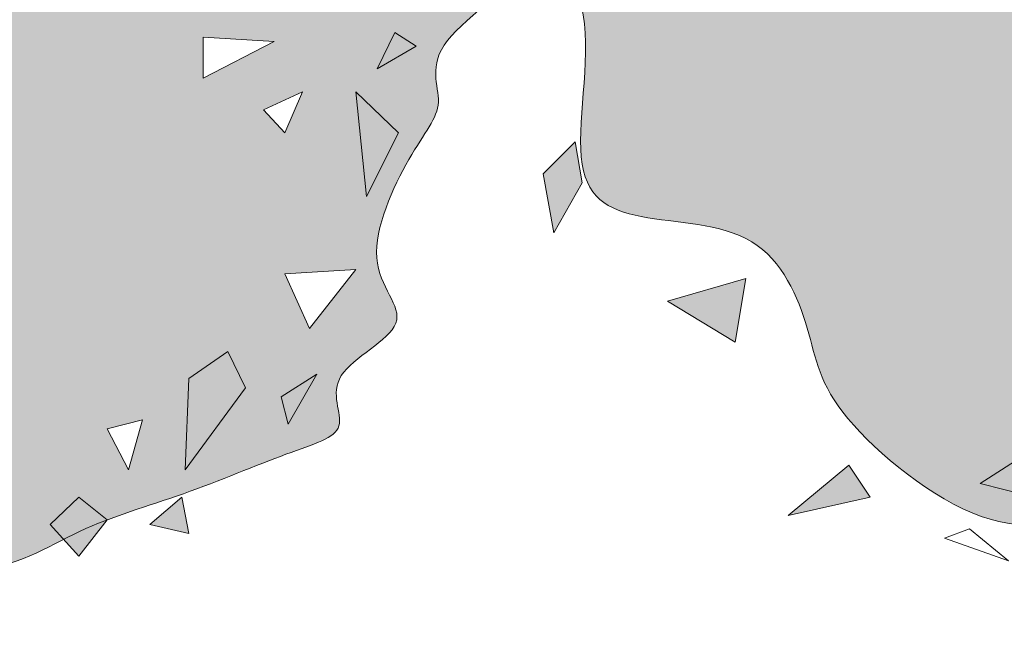
# Model space of a CAD drawing. Units: metres. Extents: x 4298.5 to 4325.2, y 2075 to 2095.8.
# Tile 6 of 35: x 4306.6693 to 4307.1445, y 2079.0337 to 2079.3365. Entities that reach past the tile are written whole.
import ezdxf

# ---------------------------------------------------------------- set-up
doc = ezdxf.new("R2010")
doc.units = ezdxf.units.M
doc.layers.add('A-ANNO-DIMS', color=2, linetype='Continuous', lineweight=18)
doc.layers.add('L-PLNT', color=94, linetype='Continuous', lineweight=13)
doc.layers.add('L-PLNT-PATT', color=116, linetype='Continuous', lineweight=13, true_color=0x13823e)
doc.styles.get("Standard").update_dxf_attribs({"font": 'arial.ttf'})
doc.dimstyles.get("Standard").update_dxf_attribs({"dimtxt": 0.18, "dimasz": 0.18, "dimexe": 0.18, "dimexo": 0.0625, "dimgap": 0.09, "dimtad": 0, "dimtih": 1, "dimtoh": 1, "dimdec": 4, "dimzin": 0, "dimdsep": 46, "dimtxsty": 'Standard', "dimcen": 0.09, "dimadec": 0, "dimazin": 0, "dimtfac": 1, "dimtdec": 4, "dimtofl": 0, "dimtmove": 0, "dimatfit": 3, "dimfxl": 1, "dimtolj": 1, "dimtzin": 0, "dimarcsym": 0})

# ---------------------------------------------------------------- blocks, each defined once
blk = doc.blocks.new('*U9')
for points in [[(7.783, -0.803), (6.433, -1.495), (6.433, -0.716)], [(10.078, -0.629), (9.74, -1.322), (10.482, -0.889)], [(8.323, -1.754), (7.985, -2.533), (7.581, -2.1)], [(9.335, -1.754), (9.538, -3.744), (10.145, -2.533)], [(-10.034, -2.706), (-10.641, -3.312), (-10.439, -4.436), (-9.899, -3.485)], [(9.335, -5.129), (8.458, -6.253), (7.985, -5.215)], [(-8.279, -5.734), (-6.794, -5.302), (-6.997, -6.513)], [(6.096, -8.935), (6.163, -7.205), (6.906, -6.686), (7.243, -7.378)], [(8.053, -8.07), (8.593, -7.118), (7.918, -7.551)], [(5.286, -7.984), (4.611, -8.157), (5.016, -8.935)], [(-2.34, -9.195), (-1.26, -8.503), (-0.99, -9.541)], [(-4.837, -8.849), (-4.432, -9.454), (-5.985, -9.801)], [(4.071, -9.454), (3.531, -9.974), (4.071, -10.579), (4.611, -9.887)], [(6.028, -9.454), (5.421, -9.974), (6.163, -10.147)], [(-2.543, -10.06), (-3.015, -10.233), (-1.8, -10.666)]]:
    blk.add_lwpolyline(points, close=True)
blk = doc.blocks.new('*D23')
at = {"layer": 'A-ANNO-DIMS', "color": 0, "lineweight": -2, "transparency": 16777216}
for p, q in [((4308.16058, 2079.85556), (4308.16058, 2079.58806)), ((4309.16058, 2079.85556), (4309.16058, 2079.58806)), ((4308.16058, 2079.76806), (4307.98058, 2079.76806)), ((4308.98058, 2079.76806), (4308.34058, 2079.76806))]:
    blk.add_line(p, q, dxfattribs=at)
at = {"layer": 'A-ANNO-DIMS', "color": 0, "transparency": 16777216}
for points in [[(4308.34058, 2079.79806), (4308.34058, 2079.73806), (4308.16058, 2079.76806)], [(4308.98058, 2079.79806), (4308.98058, 2079.73806), (4309.16058, 2079.76806)]]:
    blk.add_solid(points, dxfattribs=at)
at = {"layer": 'Defpoints', "color": 0, "transparency": 16777216}
for p in [(4308.16058, 2079.91806), (4309.16058, 2079.91806), (4308.16058, 2079.76806)]:
    blk.add_point(p, dxfattribs=at)
at = {"layer": 'A-ANNO-DIMS', "color": 0, "transparency": 16777216, "insert": (4306.70861, 2079.76806), "char_height": 0.18, "attachment_point": 5}
blk.add_mtext('\\A1;WINDOW W1 1 TYP.', dxfattribs=at)
blk = doc.blocks.new('*D47')
at = {"layer": 'A-ANNO-DIMS', "color": 0, "lineweight": -2, "transparency": 16777216}
for p, q in [((4300.43058, 2084.49556), (4300.43058, 2074.98956)), ((4322.81058, 2084.49556), (4322.81058, 2074.98956)), ((4300.61058, 2075.16956), (4311.22515, 2075.16956)), ((4322.63058, 2075.16956), (4312.016, 2075.16956))]:
    blk.add_line(p, q, dxfattribs=at)
at = {"layer": 'A-ANNO-DIMS', "color": 0, "transparency": 16777216}
for points in [[(4300.61058, 2075.19956), (4300.61058, 2075.13956), (4300.43058, 2075.16956)], [(4322.63058, 2075.19956), (4322.63058, 2075.13956), (4322.81058, 2075.16956)]]:
    blk.add_solid(points, dxfattribs=at)
at = {"layer": 'Defpoints', "color": 0, "transparency": 16777216}
for p in [(4300.43058, 2084.55806), (4322.81058, 2084.55806), (4322.81058, 2075.16956)]:
    blk.add_point(p, dxfattribs=at)
at = {"layer": 'A-ANNO-DIMS', "color": 0, "transparency": 16777216, "insert": (4311.62058, 2075.16956), "char_height": 0.18, "attachment_point": 5}
blk.add_mtext('\\A1;22.38', dxfattribs=at)
blk = doc.blocks.new('*D54')
at = {"layer": 'A-ANNO-DIMS', "color": 0, "lineweight": -2, "transparency": 16777216}
for p, q in [((4305.59808, 2079.82806), (4299.09208, 2079.82806)), ((4299.27208, 2079.64806), (4299.27208, 2078.26002)), ((4299.27208, 2076.50806), (4299.27208, 2077.89609)), ((4309.09808, 2076.32806), (4299.09208, 2076.32806))]:
    blk.add_line(p, q, dxfattribs=at)
at = {"layer": 'A-ANNO-DIMS', "color": 0, "transparency": 16777216}
for points in [[(4299.24208, 2079.64806), (4299.30208, 2079.64806), (4299.27208, 2079.82806)], [(4299.24208, 2076.50806), (4299.30208, 2076.50806), (4299.27208, 2076.32806)]]:
    blk.add_solid(points, dxfattribs=at)
at = {"layer": 'Defpoints', "color": 0, "transparency": 16777216}
for p in [(4305.66058, 2079.82806), (4299.27208, 2076.32806), (4309.16058, 2076.32806)]:
    blk.add_point(p, dxfattribs=at)
at = {"layer": 'A-ANNO-DIMS', "color": 0, "transparency": 16777216, "insert": (4299.27208, 2078.07806), "char_height": 0.18, "attachment_point": 5}
blk.add_mtext('\\A1;3.5', dxfattribs=at)
blk = doc.blocks.new('*D59')
at = {"layer": 'A-ANNO-DIMS', "color": 0, "lineweight": -2, "transparency": 16777216}
for p, q in [((4305.89058, 2079.99556), (4305.89058, 2074.98956)), ((4307.39058, 2079.99556), (4307.39058, 2074.98956)), ((4306.07058, 2075.16956), (4306.39452, 2075.16956)), ((4307.21058, 2075.16956), (4306.88663, 2075.16956))]:
    blk.add_line(p, q, dxfattribs=at)
at = {"layer": 'A-ANNO-DIMS', "color": 0, "transparency": 16777216}
for points in [[(4306.07058, 2075.19956), (4306.07058, 2075.13956), (4305.89058, 2075.16956)], [(4307.21058, 2075.19956), (4307.21058, 2075.13956), (4307.39058, 2075.16956)]]:
    blk.add_solid(points, dxfattribs=at)
at = {"layer": 'Defpoints', "color": 0, "transparency": 16777216}
for p in [(4305.89058, 2080.05806), (4307.39058, 2080.05806), (4307.39058, 2075.16956)]:
    blk.add_point(p, dxfattribs=at)
at = {"layer": 'A-ANNO-DIMS', "color": 0, "transparency": 16777216, "insert": (4306.64058, 2075.16956), "char_height": 0.18, "attachment_point": 5}
blk.add_mtext('\\A1;1.5', dxfattribs=at)
blk = doc.blocks.new('*D78')
at = {"layer": 'A-ANNO-DIMS', "color": 0, "lineweight": -2, "transparency": 16777216}
for p, q in [((4312.4969, 2079.73934), (4312.4969, 2079.91934)), ((4312.4069, 2079.82934), (4312.5869, 2079.82934)), ((4305.38467, 2076.78063), (4307.88631, 2077.85298)), ((4305.20467, 2076.78063), (4305.38467, 2076.78063))]:
    blk.add_line(p, q, dxfattribs=at)
at = {"layer": 'A-ANNO-DIMS', "color": 0, "transparency": 16777216}
blk.add_solid([(4307.87449, 2077.88055), (4307.89813, 2077.8254), (4308.05176, 2077.92389)], dxfattribs=at)
at = {"layer": 'Defpoints', "color": 0, "transparency": 16777216}
for p in [(4312.4969, 2079.82934), (4308.05176, 2077.92389)]:
    blk.add_point(p, dxfattribs=at)
at = {"layer": 'A-ANNO-DIMS', "color": 0, "transparency": 16777216, "insert": (4304.52998, 2076.78063), "char_height": 0.18, "attachment_point": 5}
blk.add_mtext('\\A1;2X R4.836', dxfattribs=at)

msp = doc.modelspace()

# ---------------------------------------------------------------- hatches: boundary and pattern name
at = {"layer": 'L-PLNT-PATT'}
h = msp.add_hatch(color=256, dxfattribs=at)
h.dxf.hatch_style = 1
edge = h.paths.add_edge_path()
edge.add_spline(control_points=[(4306.69044, 2079.08578), (4306.69302, 2079.08709), (4306.71165, 2079.09641), (4306.74745, 2079.10618), (4306.80198, 2079.12944), (4306.83132, 2079.13707), (4306.8126, 2079.16551), (4306.86518, 2079.18971), (4306.83145, 2079.21603), (4306.85847, 2079.27577), (4306.8772, 2079.29524), (4306.86058, 2079.32373), (4306.93479, 2079.3686), (4306.86486, 2079.39817), (4306.89754, 2079.40581), (4306.89356, 2079.44094), (4306.85545, 2079.47755), (4306.87404, 2079.4969), (4306.82098, 2079.54789), (4306.82098, 2079.59392), (4306.77312, 2079.5973), (4306.75268, 2079.62919), (4306.69947, 2079.62919), (4306.64714, 2079.67454), (4306.61235, 2079.63742), (4306.55167, 2079.68828), (4306.51176, 2079.61822), (4306.46721, 2079.64819), (4306.45286, 2079.60881), (4306.41256, 2079.5858), (4306.40621, 2079.58183)], knot_values=[0.818571, 0.818571, 0.818571, 0.818571, 0.97924, 1.97924, 2.97924, 3.97924, 4.97924, 5.97924, 6.97924, 7.97924, 8.97924, 9.97924, 10.97924, 11.97924, 12.97924, 13.97924, 14.97924, 15.97924, 16.97924, 17.97924, 18.97924, 19.97924, 20.97924, 21.97924, 22.97924, 23.97924, 24.97924, 25.97924, 26.97924, 27.16067, 27.16067, 27.16067, 27.16067], degree=3, periodic=0)
edge.add_line((4306.40621, 2079.58183), (4306.44747, 2079.59404))
edge.add_line((4306.44747, 2079.59404), (4306.43546, 2079.56107))
edge.add_line((4306.43546, 2079.56107), (4306.39091, 2079.53691))
edge.add_line((4306.39091, 2079.53691), (4306.40253, 2079.5795))
edge.add_spline(control_points=[(4306.40253, 2079.5795), (4306.37988, 2079.56484), (4306.35659, 2079.5439), (4306.35932, 2079.49949)], knot_values=[0.141368, 0.141368, 0.141368, 0.141368, 0.783694, 0.783694, 0.783694, 0.783694], degree=3, periodic=0)
edge.add_spline(control_points=[(4306.35932, 2079.49949), (4306.36329, 2079.49923), (4306.36753, 2079.49889), (4306.37205, 2079.49844)], knot_values=[40.901028, 40.901028, 40.901028, 40.901028, 41, 41, 41, 41], degree=3, periodic=0)
edge.add_line((4306.37205, 2079.49844), (4306.38748, 2079.49955))
edge.add_line((4306.38748, 2079.49955), (4306.36518, 2079.46658))
edge.add_line((4306.36518, 2079.46658), (4306.35662, 2079.49734))
edge.add_line((4306.35662, 2079.49734), (4306.35944, 2079.49754))
edge.add_spline(control_points=[(4306.35945, 2079.49754), (4306.3594, 2079.4982), (4306.35936, 2079.49885), (4306.35932, 2079.49949)], knot_values=[0.13204, 0.13204, 0.13204, 0.13204, 0.141368, 0.141368, 0.141368, 0.141368], degree=3, periodic=0)
edge.add_spline(control_points=[(4306.35932, 2079.49949), (4306.3231, 2079.50184), (4306.2915, 2079.49199), (4306.23947, 2079.53397), (4306.30655, 2079.43142), (4306.30887, 2079.40456), (4306.30956, 2079.39708)], knot_values=[37.439141, 37.439141, 37.439141, 37.439141, 38.340169, 39.340169, 40.340169, 40.901028, 40.901028, 40.901028, 40.901028], degree=3, periodic=0)
edge.add_line((4306.30956, 2079.39708), (4306.32919, 2079.43582))
edge.add_line((4306.32919, 2079.43582), (4306.34976, 2079.43361))
edge.add_line((4306.34976, 2079.43361), (4306.34463, 2079.40504))
edge.add_line((4306.34463, 2079.40504), (4306.30999, 2079.39293))
edge.add_spline(control_points=[(4306.30999, 2079.39293), (4306.31047, 2079.38899), (4306.31356, 2079.37544), (4306.35492, 2079.35449), (4306.33345, 2079.25721), (4306.3657, 2079.23836), (4306.43192, 2079.23836), (4306.45469, 2079.18462), (4306.45818, 2079.14915), (4306.53918, 2079.08309), (4306.59748, 2079.09986), (4306.64786, 2079.06298), (4306.677, 2079.07895), (4306.69044, 2079.08578)], knot_values=[27.16067, 27.16067, 27.16067, 27.16067, 27.490087, 28.490087, 29.490087, 30.490087, 31.490087, 32.490087, 33.490087, 34.490087, 35.490087, 36.490087, 37.329418, 37.329418, 37.329418, 37.329418], degree=3, periodic=0)
edge.add_line((4306.69044, 2079.08578), (4306.68402, 2079.09297))
edge.add_line((4306.68402, 2079.09297), (4306.69774, 2079.10618))
edge.add_line((4306.69774, 2079.10618), (4306.71147, 2079.09517))
h.paths.add_polyline_path([(4306.66688, 2079.43582), (4306.69088, 2079.43582), (4306.68402, 2079.39406)], flags=16)
h.paths.add_polyline_path([(4306.7029, 2079.41603), (4306.7286, 2079.41382), (4306.70633, 2079.37867)], flags=16)
h.paths.add_polyline_path([(4306.49548, 2079.46876), (4306.45603, 2079.45998), (4306.47834, 2079.50834)], flags=16)
h.paths.add_polyline_path([(4306.62233, 2079.49734), (4306.5966, 2079.51052), (4306.61374, 2079.5281)], flags=16)
h.paths.add_polyline_path([(4306.7029, 2079.44022), (4306.70633, 2079.46219), (4306.73373, 2079.42922)], flags=16)
h.paths.add_polyline_path([(4306.72174, 2079.3567), (4306.74232, 2079.38527), (4306.75946, 2079.3567), (4306.73373, 2079.3457)], flags=16)
h.paths.add_polyline_path([(4306.65832, 2079.49516), (4306.65832, 2079.51931), (4306.71146, 2079.51713), (4306.70633, 2079.47755)], flags=16)
h.paths.add_polyline_path([(4306.63775, 2079.50613), (4306.63775, 2079.52591), (4306.66175, 2079.53691), (4306.64803, 2079.52152)], flags=16)
h.paths.add_polyline_path([(4306.5366, 2079.51713), (4306.51433, 2079.51492), (4306.52118, 2079.53691)], flags=16)
h.paths.add_polyline_path([(4306.55032, 2079.5281), (4306.56061, 2079.56328), (4306.5949, 2079.57646), (4306.60175, 2079.54349)], flags=16)
h.paths.add_polyline_path([(4306.41661, 2079.39185), (4306.40462, 2079.35888), (4306.39261, 2079.38527)], flags=16)
h.paths.add_polyline_path([(4306.7526, 2079.40064), (4306.78517, 2079.38967), (4306.76975, 2079.37867)], flags=16)
h.paths.add_polyline_path([(4306.73203, 2079.46876), (4306.73373, 2079.48637), (4306.75088, 2079.47537)], flags=16)
h.paths.add_polyline_path([(4306.6429, 2079.54349), (4306.62919, 2079.56328), (4306.67374, 2079.56986), (4306.69088, 2079.5457)], flags=16)
h.paths.add_polyline_path([(4306.75774, 2079.32812), (4306.79203, 2079.32592), (4306.75774, 2079.30834)], flags=16)
h.paths.add_polyline_path([(4306.39434, 2079.41164), (4306.37889, 2079.40504), (4306.38575, 2079.42482)], flags=16)
h.paths.add_polyline_path([(4306.49718, 2079.5457), (4306.47148, 2079.56546), (4306.49205, 2079.57425)], flags=16)
h.paths.add_polyline_path([(4306.42863, 2079.49076), (4306.4252, 2079.50394), (4306.44747, 2079.51931)], flags=16)
h.paths.add_polyline_path([(4306.5366, 2079.56328), (4306.53147, 2079.57425), (4306.54519, 2079.58743), (4306.54862, 2079.57646)], flags=16)
h.paths.add_polyline_path([(4306.75946, 2079.45119), (4306.77488, 2079.46437), (4306.80058, 2079.47316), (4306.7886, 2079.44461), (4306.80058, 2079.43582), (4306.78174, 2079.42482)], flags=16)
h.paths.add_polyline_path([(4306.38575, 2079.3567), (4306.35492, 2079.35449), (4306.34463, 2079.36767)], flags=16)
h.paths.add_polyline_path([(4306.73546, 2079.50394), (4306.73373, 2079.54128), (4306.75774, 2079.54789), (4306.75946, 2079.51492)], flags=16)
h.paths.add_polyline_path([(4306.78517, 2079.3501), (4306.80058, 2079.36549), (4306.82632, 2079.35888), (4306.82116, 2079.33912)], flags=16)
h.paths.add_polyline_path([(4306.70975, 2079.54349), (4306.71146, 2079.55667), (4306.72004, 2079.55667), (4306.72004, 2079.5391)], flags=16)
h.paths.add_polyline_path([(4306.63604, 2079.58085), (4306.64117, 2079.59404), (4306.66002, 2079.59843), (4306.65316, 2079.58525)], flags=16)
h.paths.add_polyline_path([(4306.79545, 2079.39846), (4306.80231, 2079.41164), (4306.8143, 2079.38527)], flags=16)
h.paths.add_polyline_path([(4306.78689, 2079.29297), (4306.80574, 2079.30176), (4306.79716, 2079.28197)], flags=16)
h.paths.add_polyline_path([(4306.58118, 2079.60283), (4306.55375, 2079.61601), (4306.54346, 2079.64237), (4306.57432, 2079.6248), (4306.58974, 2079.61601)], flags=16)
h.paths.add_polyline_path([(4306.61374, 2079.60064), (4306.60861, 2079.63359), (4306.62576, 2079.65119), (4306.65832, 2079.62701)], flags=16)
h.paths.add_polyline_path([(4306.49375, 2079.58743), (4306.46289, 2079.60943), (4306.48176, 2079.62701), (4306.54176, 2079.60943)], flags=16)
h.paths.add_polyline_path([(4306.77661, 2079.50394), (4306.79375, 2079.51931), (4306.83145, 2079.50834), (4306.82289, 2079.48637)], flags=16)
h.paths.add_polyline_path([(4306.69604, 2079.58085), (4306.68575, 2079.60064), (4306.69947, 2079.62919), (4306.71146, 2079.60064), (4306.72345, 2079.60504), (4306.75431, 2079.58525), (4306.72687, 2079.56767)], flags=16)
h.paths.add_polyline_path([(4306.80744, 2079.44461), (4306.80231, 2079.46219), (4306.81603, 2079.46658), (4306.8126, 2079.449)], flags=16)
h.paths.add_polyline_path([(4306.82289, 2079.40504), (4306.82802, 2079.449), (4306.85545, 2079.47755), (4306.85545, 2079.41822), (4306.83145, 2079.40725), (4306.85718, 2079.40943), (4306.89317, 2079.3567), (4306.86058, 2079.35888)], flags=16)
h.paths.add_polyline_path([(4306.56233, 2079.13034), (4306.56919, 2079.10397), (4306.5349, 2079.11276)], flags=16)
h.paths.add_polyline_path([(4306.77488, 2079.54789), (4306.78347, 2079.58304), (4306.81087, 2079.54789)], flags=16)
h.paths.add_polyline_path([(4306.83145, 2079.30176), (4306.85202, 2079.28197), (4306.8366, 2079.25121)], flags=16)
h.paths.add_polyline_path([(4306.84173, 2079.31273), (4306.85032, 2079.33033), (4306.86058, 2079.32373)], flags=16)
h.paths.add_polyline_path([(4306.71146, 2079.13912), (4306.7286, 2079.14352), (4306.72174, 2079.11936)], flags=16)
h.paths.add_polyline_path([(4306.79716, 2079.21385), (4306.83145, 2079.21603), (4306.80917, 2079.18749)], flags=16)
h.paths.add_polyline_path([(4306.75088, 2079.1633), (4306.76975, 2079.17649), (4306.77831, 2079.15891), (4306.74918, 2079.11936)], flags=16)
h.paths.add_polyline_path([(4306.79545, 2079.15452), (4306.8126, 2079.16551), (4306.79888, 2079.14133)], flags=16)
h = msp.add_hatch(color=256, dxfattribs=at)
h.dxf.hatch_style = 1
edge = h.paths.add_edge_path()
edge.add_spline(control_points=[(4307.28832, 2079.08578), (4307.29089, 2079.08709), (4307.30952, 2079.09641), (4307.34532, 2079.10618), (4307.39985, 2079.12944), (4307.4292, 2079.13707), (4307.41047, 2079.16551), (4307.46306, 2079.18971), (4307.42932, 2079.21603), (4307.45635, 2079.27577), (4307.47508, 2079.29524), (4307.45845, 2079.32373), (4307.53267, 2079.3686), (4307.46273, 2079.39817), (4307.49542, 2079.40581), (4307.49143, 2079.44094), (4307.45332, 2079.47755), (4307.47191, 2079.4969), (4307.41885, 2079.54789), (4307.41885, 2079.59392), (4307.37099, 2079.5973), (4307.35056, 2079.62919), (4307.29734, 2079.62919), (4307.24502, 2079.67454), (4307.21022, 2079.63742), (4307.14954, 2079.68828), (4307.10964, 2079.61822), (4307.06508, 2079.64819), (4307.05073, 2079.60881), (4307.01044, 2079.5858), (4307.00408, 2079.58183)], knot_values=[0.818571, 0.818571, 0.818571, 0.818571, 0.97924, 1.97924, 2.97924, 3.97924, 4.97924, 5.97924, 6.97924, 7.97924, 8.97924, 9.97924, 10.97924, 11.97924, 12.97924, 13.97924, 14.97924, 15.97924, 16.97924, 17.97924, 18.97924, 19.97924, 20.97924, 21.97924, 22.97924, 23.97924, 24.97924, 25.97924, 26.97924, 27.16067, 27.16067, 27.16067, 27.16067], degree=3, periodic=0)
edge.add_line((4307.00408, 2079.58183), (4307.04535, 2079.59404))
edge.add_line((4307.04535, 2079.59404), (4307.03333, 2079.56107))
edge.add_line((4307.03333, 2079.56107), (4306.98878, 2079.53691))
edge.add_line((4306.98878, 2079.53691), (4307.0004, 2079.5795))
edge.add_spline(control_points=[(4307.0004, 2079.5795), (4306.97776, 2079.56484), (4306.95447, 2079.5439), (4306.95719, 2079.49949)], knot_values=[0.141368, 0.141368, 0.141368, 0.141368, 0.783694, 0.783694, 0.783694, 0.783694], degree=3, periodic=0)
edge.add_spline(control_points=[(4306.95719, 2079.49949), (4306.96117, 2079.49923), (4306.9654, 2079.49889), (4306.96992, 2079.49844)], knot_values=[40.901028, 40.901028, 40.901028, 40.901028, 41, 41, 41, 41], degree=3, periodic=0)
edge.add_line((4306.96992, 2079.49844), (4306.98535, 2079.49955))
edge.add_line((4306.98535, 2079.49955), (4306.96305, 2079.46658))
edge.add_line((4306.96305, 2079.46658), (4306.95449, 2079.49734))
edge.add_line((4306.95449, 2079.49734), (4306.95732, 2079.49754))
edge.add_spline(control_points=[(4306.95733, 2079.49754), (4306.95728, 2079.4982), (4306.95723, 2079.49885), (4306.95719, 2079.49949)], knot_values=[0.13204, 0.13204, 0.13204, 0.13204, 0.141368, 0.141368, 0.141368, 0.141368], degree=3, periodic=0)
edge.add_spline(control_points=[(4306.95719, 2079.49949), (4306.92097, 2079.50184), (4306.88937, 2079.49199), (4306.83734, 2079.53397), (4306.90442, 2079.43142), (4306.90674, 2079.40456), (4306.90744, 2079.39708)], knot_values=[37.439141, 37.439141, 37.439141, 37.439141, 38.340169, 39.340169, 40.340169, 40.901028, 40.901028, 40.901028, 40.901028], degree=3, periodic=0)
edge.add_line((4306.90744, 2079.39708), (4306.92706, 2079.43582))
edge.add_line((4306.92706, 2079.43582), (4306.94764, 2079.43361))
edge.add_line((4306.94764, 2079.43361), (4306.9425, 2079.40504))
edge.add_line((4306.9425, 2079.40504), (4306.90786, 2079.39293))
edge.add_spline(control_points=[(4306.90786, 2079.39293), (4306.90835, 2079.38899), (4306.91143, 2079.37544), (4306.95279, 2079.35449), (4306.93133, 2079.25721), (4306.96358, 2079.23836), (4307.0298, 2079.23836), (4307.05256, 2079.18462), (4307.05606, 2079.14915), (4307.13706, 2079.08309), (4307.19535, 2079.09986), (4307.24573, 2079.06298), (4307.27487, 2079.07895), (4307.28832, 2079.08578)], knot_values=[27.16067, 27.16067, 27.16067, 27.16067, 27.490087, 28.490087, 29.490087, 30.490087, 31.490087, 32.490087, 33.490087, 34.490087, 35.490087, 36.490087, 37.329418, 37.329418, 37.329418, 37.329418], degree=3, periodic=0)
edge.add_line((4307.28832, 2079.08578), (4307.2819, 2079.09297))
edge.add_line((4307.2819, 2079.09297), (4307.29562, 2079.10618))
edge.add_line((4307.29562, 2079.10618), (4307.30934, 2079.09517))
h.paths.add_polyline_path([(4307.26475, 2079.43582), (4307.28876, 2079.43582), (4307.2819, 2079.39406)], flags=16)
h.paths.add_polyline_path([(4307.30077, 2079.41603), (4307.32648, 2079.41382), (4307.3042, 2079.37867)], flags=16)
h.paths.add_polyline_path([(4307.09335, 2079.46876), (4307.05391, 2079.45998), (4307.07621, 2079.50834)], flags=16)
h.paths.add_polyline_path([(4307.2202, 2079.49734), (4307.19447, 2079.51052), (4307.21162, 2079.5281)], flags=16)
h.paths.add_polyline_path([(4307.30077, 2079.44022), (4307.3042, 2079.46219), (4307.33161, 2079.42922)], flags=16)
h.paths.add_polyline_path([(4307.31962, 2079.3567), (4307.34019, 2079.38527), (4307.35734, 2079.3567), (4307.33161, 2079.3457)], flags=16)
h.paths.add_polyline_path([(4307.25619, 2079.49516), (4307.25619, 2079.51931), (4307.30933, 2079.51713), (4307.3042, 2079.47755)], flags=16)
h.paths.add_polyline_path([(4307.23562, 2079.50613), (4307.23562, 2079.52591), (4307.25962, 2079.53691), (4307.24591, 2079.52152)], flags=16)
h.paths.add_polyline_path([(4307.13448, 2079.51713), (4307.1122, 2079.51492), (4307.11906, 2079.53691)], flags=16)
h.paths.add_polyline_path([(4307.14819, 2079.5281), (4307.15848, 2079.56328), (4307.19277, 2079.57646), (4307.19963, 2079.54349)], flags=16)
h.paths.add_polyline_path([(4307.01449, 2079.39185), (4307.0025, 2079.35888), (4306.99048, 2079.38527)], flags=16)
h.paths.add_polyline_path([(4307.35048, 2079.40064), (4307.38304, 2079.38967), (4307.36762, 2079.37867)], flags=16)
h.paths.add_polyline_path([(4307.32991, 2079.46876), (4307.33161, 2079.48637), (4307.34875, 2079.47537)], flags=16)
h.paths.add_polyline_path([(4307.24078, 2079.54349), (4307.22706, 2079.56328), (4307.27161, 2079.56986), (4307.28876, 2079.5457)], flags=16)
h.paths.add_polyline_path([(4307.35561, 2079.32812), (4307.3899, 2079.32592), (4307.35561, 2079.30834)], flags=16)
h.paths.add_polyline_path([(4306.99221, 2079.41164), (4306.97677, 2079.40504), (4306.98363, 2079.42482)], flags=16)
h.paths.add_polyline_path([(4307.09506, 2079.5457), (4307.06935, 2079.56546), (4307.08993, 2079.57425)], flags=16)
h.paths.add_polyline_path([(4307.0265, 2079.49076), (4307.02307, 2079.50394), (4307.04535, 2079.51931)], flags=16)
h.paths.add_polyline_path([(4307.13448, 2079.56328), (4307.12935, 2079.57425), (4307.14306, 2079.58743), (4307.14649, 2079.57646)], flags=16)
h.paths.add_polyline_path([(4307.35734, 2079.45119), (4307.37275, 2079.46437), (4307.39846, 2079.47316), (4307.38647, 2079.44461), (4307.39846, 2079.43582), (4307.37961, 2079.42482)], flags=16)
h.paths.add_polyline_path([(4306.98363, 2079.3567), (4306.95279, 2079.35449), (4306.9425, 2079.36767)], flags=16)
h.paths.add_polyline_path([(4307.33333, 2079.50394), (4307.33161, 2079.54128), (4307.35561, 2079.54789), (4307.35734, 2079.51492)], flags=16)
h.paths.add_polyline_path([(4307.38304, 2079.3501), (4307.39846, 2079.36549), (4307.42419, 2079.35888), (4307.41903, 2079.33912)], flags=16)
h.paths.add_polyline_path([(4307.30763, 2079.54349), (4307.30933, 2079.55667), (4307.31792, 2079.55667), (4307.31792, 2079.5391)], flags=16)
h.paths.add_polyline_path([(4307.23392, 2079.58085), (4307.23905, 2079.59404), (4307.2579, 2079.59843), (4307.25104, 2079.58525)], flags=16)
h.paths.add_polyline_path([(4307.39333, 2079.39846), (4307.40019, 2079.41164), (4307.41218, 2079.38527)], flags=16)
h.paths.add_polyline_path([(4307.38477, 2079.29297), (4307.40362, 2079.30176), (4307.39503, 2079.28197)], flags=16)
h.paths.add_polyline_path([(4307.17905, 2079.60283), (4307.15162, 2079.61601), (4307.14134, 2079.64237), (4307.1722, 2079.6248), (4307.18761, 2079.61601)], flags=16)
h.paths.add_polyline_path([(4307.21162, 2079.60064), (4307.20649, 2079.63359), (4307.22363, 2079.65119), (4307.25619, 2079.62701)], flags=16)
h.paths.add_polyline_path([(4307.09163, 2079.58743), (4307.06077, 2079.60943), (4307.07964, 2079.62701), (4307.13963, 2079.60943)], flags=16)
h.paths.add_polyline_path([(4307.37448, 2079.50394), (4307.39163, 2079.51931), (4307.42932, 2079.50834), (4307.42076, 2079.48637)], flags=16)
h.paths.add_polyline_path([(4307.29391, 2079.58085), (4307.28363, 2079.60064), (4307.29734, 2079.62919), (4307.30933, 2079.60064), (4307.32132, 2079.60504), (4307.35218, 2079.58525), (4307.32475, 2079.56767)], flags=16)
h.paths.add_polyline_path([(4307.40532, 2079.44461), (4307.40019, 2079.46219), (4307.4139, 2079.46658), (4307.41047, 2079.449)], flags=16)
h.paths.add_polyline_path([(4307.42076, 2079.40504), (4307.42589, 2079.449), (4307.45332, 2079.47755), (4307.45332, 2079.41822), (4307.42932, 2079.40725), (4307.45505, 2079.40943), (4307.49104, 2079.3567), (4307.45845, 2079.35888)], flags=16)
h.paths.add_polyline_path([(4307.16021, 2079.13034), (4307.16707, 2079.10397), (4307.13278, 2079.11276)], flags=16)
h.paths.add_polyline_path([(4307.37275, 2079.54789), (4307.38134, 2079.58304), (4307.40875, 2079.54789)], flags=16)
h.paths.add_polyline_path([(4307.42932, 2079.30176), (4307.44989, 2079.28197), (4307.43448, 2079.25121)], flags=16)
h.paths.add_polyline_path([(4307.43961, 2079.31273), (4307.44819, 2079.33033), (4307.45845, 2079.32373)], flags=16)
h.paths.add_polyline_path([(4307.30933, 2079.13912), (4307.32648, 2079.14352), (4307.31962, 2079.11936)], flags=16)
h.paths.add_polyline_path([(4307.39503, 2079.21385), (4307.42932, 2079.21603), (4307.40704, 2079.18749)], flags=16)
h.paths.add_polyline_path([(4307.34875, 2079.1633), (4307.36762, 2079.17649), (4307.37618, 2079.15891), (4307.34705, 2079.11936)], flags=16)
h.paths.add_polyline_path([(4307.39333, 2079.15452), (4307.41047, 2079.16551), (4307.39676, 2079.14133)], flags=16)
h = msp.add_hatch(color=256, dxfattribs=at)
h.dxf.hatch_style = 1
h.paths.add_polyline_path([(4306.70633, 2079.47755), (4306.71146, 2079.51713), (4306.65832, 2079.51931), (4306.65832, 2079.49516)])
h.paths.add_polyline_path([(4306.7526, 2079.40064), (4306.76975, 2079.37867), (4306.78517, 2079.38967)])
h.paths.add_polyline_path([(4306.73373, 2079.54128), (4306.73546, 2079.50394), (4306.75946, 2079.51492), (4306.75774, 2079.54789)])
h.paths.add_polyline_path([(4306.75431, 2079.58525), (4306.72345, 2079.60504), (4306.71146, 2079.60064), (4306.69947, 2079.62919), (4306.68575, 2079.60064), (4306.69604, 2079.58085), (4306.72687, 2079.56767)])
h.paths.add_polyline_path([(4306.60003, 2079.0776), (4306.61547, 2079.06), (4306.66002, 2079.05782)])
h.paths.add_polyline_path([(4306.58118, 2079.60283), (4306.58974, 2079.61601), (4306.57432, 2079.6248), (4306.54346, 2079.64237), (4306.55375, 2079.61601)])
h.paths.add_polyline_path([(4306.48176, 2079.62701), (4306.46289, 2079.60943), (4306.49375, 2079.58743), (4306.54176, 2079.60943)])
h.paths.add_polyline_path([(4306.56061, 2079.56328), (4306.55032, 2079.5281), (4306.60175, 2079.54349), (4306.5949, 2079.57646)])
h.paths.add_polyline_path([(4306.54862, 2079.57646), (4306.54519, 2079.58743), (4306.53147, 2079.57425), (4306.5366, 2079.56328)])
h.paths.add_polyline_path([(4306.52118, 2079.53691), (4306.51433, 2079.51492), (4306.5366, 2079.51713)])
h.paths.add_polyline_path([(4306.49718, 2079.5457), (4306.49205, 2079.57425), (4306.47148, 2079.56546)])
h.paths.add_polyline_path([(4306.4029, 2079.58085), (4306.39091, 2079.53691), (4306.43546, 2079.56107), (4306.44747, 2079.59404)])
h.paths.add_polyline_path([(4306.44747, 2079.51931), (4306.4252, 2079.50394), (4306.42863, 2079.49076)])
h.paths.add_polyline_path([(4306.35662, 2079.49734), (4306.36518, 2079.46658), (4306.38748, 2079.49955)])
h.paths.add_polyline_path([(4306.30691, 2079.39185), (4306.34463, 2079.40504), (4306.34976, 2079.43361), (4306.32919, 2079.43582)])
h.paths.add_polyline_path([(4306.41661, 2079.39185), (4306.39261, 2079.38527), (4306.40462, 2079.35888)])
h.paths.add_polyline_path([(4306.3429, 2079.25779), (4306.33947, 2079.27758), (4306.32406, 2079.26219), (4306.32919, 2079.23364)])
h.paths.add_polyline_path([(4306.42177, 2079.21164), (4306.38405, 2079.20067), (4306.41661, 2079.18088)])
h.paths.add_polyline_path([(4306.44232, 2079.09737), (4306.48176, 2079.10618), (4306.47148, 2079.12155)])
h.paths.add_polyline_path([(4306.56233, 2079.13034), (4306.5349, 2079.11276), (4306.56919, 2079.10397)])
h.paths.add_polyline_path([(4306.69774, 2079.10618), (4306.68402, 2079.09297), (4306.69774, 2079.0776), (4306.71146, 2079.09518)])
h.paths.add_polyline_path([(4306.77831, 2079.15891), (4306.76975, 2079.17649), (4306.75088, 2079.1633), (4306.74918, 2079.11936)])
h.paths.add_polyline_path([(4306.74745, 2079.10618), (4306.73203, 2079.09297), (4306.75088, 2079.08858)])
h.paths.add_polyline_path([(4306.79545, 2079.15452), (4306.79888, 2079.14133), (4306.8126, 2079.16551)])
h.paths.add_polyline_path([(4306.8366, 2079.25121), (4306.85202, 2079.28197), (4306.83145, 2079.30176)])
h.paths.add_polyline_path([(4306.72174, 2079.3567), (4306.73373, 2079.3457), (4306.75946, 2079.3567), (4306.74232, 2079.38527)])
h.paths.add_polyline_path([(4306.86058, 2079.35888), (4306.89317, 2079.3567), (4306.85718, 2079.40943), (4306.83145, 2079.40725), (4306.85545, 2079.41822), (4306.85545, 2079.47755), (4306.82802, 2079.449), (4306.82289, 2079.40504)])
h.paths.add_polyline_path([(4306.80058, 2079.36549), (4306.78517, 2079.3501), (4306.82116, 2079.33912), (4306.82632, 2079.35888)])
h.paths.add_polyline_path([(4306.86058, 2079.32373), (4306.85032, 2079.33033), (4306.84173, 2079.31273)])
h.paths.add_polyline_path([(4306.80058, 2079.47316), (4306.77488, 2079.46437), (4306.75946, 2079.45119), (4306.78174, 2079.42482), (4306.80058, 2079.43582), (4306.7886, 2079.44461)])
h.paths.add_polyline_path([(4306.80231, 2079.46219), (4306.80744, 2079.44461), (4306.8126, 2079.449), (4306.81603, 2079.46658)])
h.paths.add_polyline_path([(4306.82289, 2079.48637), (4306.83145, 2079.50834), (4306.79375, 2079.51931), (4306.77661, 2079.50394)])
h.paths.add_polyline_path([(4306.73373, 2079.42922), (4306.70633, 2079.46219), (4306.7029, 2079.44022)])
h.paths.add_polyline_path([(4306.69088, 2079.43582), (4306.66688, 2079.43582), (4306.68402, 2079.39406)])
h.paths.add_polyline_path([(4306.7286, 2079.41382), (4306.7029, 2079.41603), (4306.70633, 2079.37867)])
h.paths.add_polyline_path([(4306.69088, 2079.5457), (4306.67374, 2079.56986), (4306.62919, 2079.56328), (4306.6429, 2079.54349)])
h.paths.add_polyline_path([(4306.64803, 2079.52152), (4306.66175, 2079.53691), (4306.63775, 2079.52591), (4306.63775, 2079.50613)])
h.paths.add_polyline_path([(4306.61374, 2079.5281), (4306.5966, 2079.51052), (4306.62233, 2079.49734)])
h.paths.add_polyline_path([(4306.65316, 2079.58525), (4306.66002, 2079.59843), (4306.64117, 2079.59404), (4306.63604, 2079.58085)])
h.paths.add_polyline_path([(4306.78347, 2079.58304), (4306.77488, 2079.54789), (4306.81087, 2079.54789)])
h = msp.add_hatch(color=256, dxfattribs=at)
h.dxf.hatch_style = 1
h.paths.add_polyline_path([(4307.3042, 2079.47755), (4307.30933, 2079.51713), (4307.25619, 2079.51931), (4307.25619, 2079.49516)])
h.paths.add_polyline_path([(4307.35048, 2079.40064), (4307.36762, 2079.37867), (4307.38304, 2079.38967)])
h.paths.add_polyline_path([(4307.33161, 2079.54128), (4307.33333, 2079.50394), (4307.35734, 2079.51492), (4307.35561, 2079.54789)])
h.paths.add_polyline_path([(4307.35218, 2079.58525), (4307.32132, 2079.60504), (4307.30933, 2079.60064), (4307.29734, 2079.62919), (4307.28363, 2079.60064), (4307.29391, 2079.58085), (4307.32475, 2079.56767)])
h.paths.add_polyline_path([(4307.1979, 2079.0776), (4307.21334, 2079.06), (4307.2579, 2079.05782)])
h.paths.add_polyline_path([(4307.17905, 2079.60283), (4307.18761, 2079.61601), (4307.1722, 2079.6248), (4307.14134, 2079.64237), (4307.15162, 2079.61601)])
h.paths.add_polyline_path([(4307.07964, 2079.62701), (4307.06077, 2079.60943), (4307.09163, 2079.58743), (4307.13963, 2079.60943)])
h.paths.add_polyline_path([(4307.15848, 2079.56328), (4307.14819, 2079.5281), (4307.19963, 2079.54349), (4307.19277, 2079.57646)])
h.paths.add_polyline_path([(4307.14649, 2079.57646), (4307.14306, 2079.58743), (4307.12935, 2079.57425), (4307.13448, 2079.56328)])
h.paths.add_polyline_path([(4307.11906, 2079.53691), (4307.1122, 2079.51492), (4307.13448, 2079.51713)])
h.paths.add_polyline_path([(4307.09506, 2079.5457), (4307.08993, 2079.57425), (4307.06935, 2079.56546)])
h.paths.add_polyline_path([(4307.00077, 2079.58085), (4306.98878, 2079.53691), (4307.03333, 2079.56107), (4307.04535, 2079.59404)])
h.paths.add_polyline_path([(4307.04535, 2079.51931), (4307.02307, 2079.50394), (4307.0265, 2079.49076)])
h.paths.add_polyline_path([(4306.95449, 2079.49734), (4306.96305, 2079.46658), (4306.98535, 2079.49955)])
h.paths.add_polyline_path([(4306.90479, 2079.39185), (4306.9425, 2079.40504), (4306.94764, 2079.43361), (4306.92706, 2079.43582)])
h.paths.add_polyline_path([(4307.01449, 2079.39185), (4306.99048, 2079.38527), (4307.0025, 2079.35888)])
h.paths.add_polyline_path([(4306.94078, 2079.25779), (4306.93735, 2079.27758), (4306.92193, 2079.26219), (4306.92706, 2079.23364)])
h.paths.add_polyline_path([(4307.01964, 2079.21164), (4306.98193, 2079.20067), (4307.01449, 2079.18088)])
h.paths.add_polyline_path([(4307.04019, 2079.09737), (4307.07964, 2079.10618), (4307.06935, 2079.12155)])
h.paths.add_polyline_path([(4307.16021, 2079.13034), (4307.13278, 2079.11276), (4307.16707, 2079.10397)])
h.paths.add_polyline_path([(4307.29562, 2079.10618), (4307.2819, 2079.09297), (4307.29562, 2079.0776), (4307.30933, 2079.09518)])
h.paths.add_polyline_path([(4307.37618, 2079.15891), (4307.36762, 2079.17649), (4307.34875, 2079.1633), (4307.34705, 2079.11936)])
h.paths.add_polyline_path([(4307.34532, 2079.10618), (4307.32991, 2079.09297), (4307.34875, 2079.08858)])
h.paths.add_polyline_path([(4307.39333, 2079.15452), (4307.39676, 2079.14133), (4307.41047, 2079.16551)])
h.paths.add_polyline_path([(4307.43448, 2079.25121), (4307.44989, 2079.28197), (4307.42932, 2079.30176)])
h.paths.add_polyline_path([(4307.31962, 2079.3567), (4307.33161, 2079.3457), (4307.35734, 2079.3567), (4307.34019, 2079.38527)])
h.paths.add_polyline_path([(4307.45845, 2079.35888), (4307.49104, 2079.3567), (4307.45505, 2079.40943), (4307.42932, 2079.40725), (4307.45332, 2079.41822), (4307.45332, 2079.47755), (4307.42589, 2079.449), (4307.42076, 2079.40504)])
h.paths.add_polyline_path([(4307.39846, 2079.36549), (4307.38304, 2079.3501), (4307.41903, 2079.33912), (4307.42419, 2079.35888)])
h.paths.add_polyline_path([(4307.45845, 2079.32373), (4307.44819, 2079.33033), (4307.43961, 2079.31273)])
h.paths.add_polyline_path([(4307.39846, 2079.47316), (4307.37275, 2079.46437), (4307.35734, 2079.45119), (4307.37961, 2079.42482), (4307.39846, 2079.43582), (4307.38647, 2079.44461)])
h.paths.add_polyline_path([(4307.40019, 2079.46219), (4307.40532, 2079.44461), (4307.41047, 2079.449), (4307.4139, 2079.46658)])
h.paths.add_polyline_path([(4307.42076, 2079.48637), (4307.42932, 2079.50834), (4307.39163, 2079.51931), (4307.37448, 2079.50394)])
h.paths.add_polyline_path([(4307.33161, 2079.42922), (4307.3042, 2079.46219), (4307.30077, 2079.44022)])
h.paths.add_polyline_path([(4307.28876, 2079.43582), (4307.26475, 2079.43582), (4307.2819, 2079.39406)])
h.paths.add_polyline_path([(4307.32648, 2079.41382), (4307.30077, 2079.41603), (4307.3042, 2079.37867)])
h.paths.add_polyline_path([(4307.28876, 2079.5457), (4307.27161, 2079.56986), (4307.22706, 2079.56328), (4307.24078, 2079.54349)])
h.paths.add_polyline_path([(4307.24591, 2079.52152), (4307.25962, 2079.53691), (4307.23562, 2079.52591), (4307.23562, 2079.50613)])
h.paths.add_polyline_path([(4307.21162, 2079.5281), (4307.19447, 2079.51052), (4307.2202, 2079.49734)])
h.paths.add_polyline_path([(4307.25104, 2079.58525), (4307.2579, 2079.59843), (4307.23905, 2079.59404), (4307.23392, 2079.58085)])
h.paths.add_polyline_path([(4307.38134, 2079.58304), (4307.37275, 2079.54789), (4307.40875, 2079.54789)])

# ---------------------------------------------------------------- linework, layer by layer
at = {"layer": 'L-PLNT'}
for points in [[(4306.36518, 2079.46658), (4306.3411, 2079.55309), (4306.44747, 2079.59404), (4306.46721, 2079.64819), (4306.51176, 2079.61822), (4306.55167, 2079.68828), (4306.61235, 2079.63742), (4306.64714, 2079.67454), (4306.69947, 2079.62919), (4306.75268, 2079.62919), (4306.77312, 2079.5973), (4306.82098, 2079.59392), (4306.82098, 2079.54789), (4306.87404, 2079.4969), (4306.85545, 2079.47755), (4306.89356, 2079.44094), (4306.89754, 2079.40581), (4306.86486, 2079.39817), (4306.93479, 2079.3686), (4306.86058, 2079.32373), (4306.8772, 2079.29524), (4306.85847, 2079.27577), (4306.83145, 2079.21603), (4306.86518, 2079.18971), (4306.8126, 2079.16551), (4306.83132, 2079.13707), (4306.80198, 2079.12944), (4306.74745, 2079.10618), (4306.69774, 2079.09262), (4306.65071, 2079.06089), (4306.59748, 2079.09986), (4306.53918, 2079.08309), (4306.45818, 2079.14915), (4306.45469, 2079.18462), (4306.43192, 2079.23836), (4306.3657, 2079.23836), (4306.33345, 2079.25721), (4306.35492, 2079.35449), (4306.30165, 2079.38148), (4306.31805, 2079.41384), (4306.23947, 2079.53397), (4306.29327, 2079.49056), (4306.32638, 2079.50297), (4306.37205, 2079.49844)], [(4306.96305, 2079.46658), (4306.93898, 2079.55309), (4307.04535, 2079.59404), (4307.06508, 2079.64819), (4307.10964, 2079.61822), (4307.14954, 2079.68828), (4307.21022, 2079.63742), (4307.24502, 2079.67454), (4307.29734, 2079.62919), (4307.35056, 2079.62919), (4307.37099, 2079.5973), (4307.41885, 2079.59392), (4307.41885, 2079.54789), (4307.47191, 2079.4969), (4307.45332, 2079.47755), (4307.49143, 2079.44094), (4307.49542, 2079.40581), (4307.46273, 2079.39817), (4307.53267, 2079.3686), (4307.45845, 2079.32373), (4307.47508, 2079.29524), (4307.45635, 2079.27577), (4307.42932, 2079.21603), (4307.46306, 2079.18971), (4307.41047, 2079.16551), (4307.4292, 2079.13707), (4307.39985, 2079.12944), (4307.34532, 2079.10618), (4307.29562, 2079.09262), (4307.24858, 2079.06089), (4307.19535, 2079.09986), (4307.13706, 2079.08309), (4307.05606, 2079.14915), (4307.05256, 2079.18462), (4307.0298, 2079.23836), (4306.96358, 2079.23836), (4306.93133, 2079.25721), (4306.95279, 2079.35449), (4306.89953, 2079.38148), (4306.91592, 2079.41384), (4306.83734, 2079.53397), (4306.89115, 2079.49056), (4306.92426, 2079.50297), (4306.96992, 2079.49844)]]:
    msp.add_open_spline(points, degree=3, dxfattribs=at)

# ---------------------------------------------------------------- block references
at = {"layer": 'L-PLNT', "xscale": 0.0254, "yscale": 0.0254, "zscale": 0.0254}
for p in [(4306.59434, 2079.34632), (4307.19222, 2079.34632)]:
    msp.add_blockref('*U9', p, dxfattribs=at)

# ---------------------------------------------------------------- dimensions: what is measured, and where the dimension line sits
at = {"layer": 'A-ANNO-DIMS'}
for base, p1, p2, override, picture, middle in [((4322.81058, 2075.16956), (4300.43058, 2084.55806), (4322.81058, 2084.55806), {"dimdec": 2, "dimlfac": 1, "dimrnd": 0, "dimzin": 0, "dimdsep": 46, "dimlunit": 2}, '*D47', (4311.62058, 2075.16956)), ((4307.39058, 2075.16956), (4305.89058, 2080.05806), (4307.39058, 2080.05806), {"dimdec": 1, "dimlfac": 1, "dimrnd": 0, "dimzin": 0, "dimdsep": 46, "dimlunit": 2}, '*D59', (4306.64058, 2075.16956))]:
    dim = msp.add_linear_dim(base=base, p1=p1, p2=p2, dimstyle='Standard', override=override, dxfattribs=at)
    dim.commit()
    dim.dimension.update_dxf_attribs({"geometry": picture, "text_midpoint": middle})
dim = msp.add_linear_dim(base=(4308.16058, 2079.76806), p1=(4309.16058, 2079.91806), p2=(4308.16058, 2079.91806), angle=180, text='WINDOW W1 <> TYP.', dimstyle='Standard', override={"dimdec": 0, "dimlfac": 1, "dimrnd": 0, "dimzin": 0, "dimdsep": 46, "dimlunit": 2}, dxfattribs=at)
dim.commit()
dim.dimension.update_dxf_attribs({"geometry": '*D23', "text_midpoint": (4306.70861, 2079.76806)})
dim = msp.add_radius_dim(center=(4312.4969, 2079.82934), mpoint=(4308.05176, 2077.92389), text='2X <>', dimstyle='Standard', override={"dimdec": 3, "dimlfac": 1, "dimrnd": 0, "dimzin": 0, "dimdsep": 46, "dimlunit": 2}, dxfattribs=at)
dim.commit()
dim.dimension.update_dxf_attribs({"geometry": '*D78', "text_midpoint": (4304.52998, 2076.78063), "dimtype": 164})
dim = msp.add_linear_dim(base=(4299.27208, 2076.32806), p1=(4305.66058, 2079.82806), p2=(4309.16058, 2076.32806), angle=90, dimstyle='Standard', override={"dimdec": 1, "dimlfac": 1, "dimrnd": 0, "dimzin": 0, "dimdsep": 46, "dimlunit": 2}, dxfattribs=at)
dim.commit()
dim.dimension.update_dxf_attribs({"geometry": '*D54', "text_midpoint": (4299.27208, 2078.07806)})

doc.saveas('drawing.dxf')
